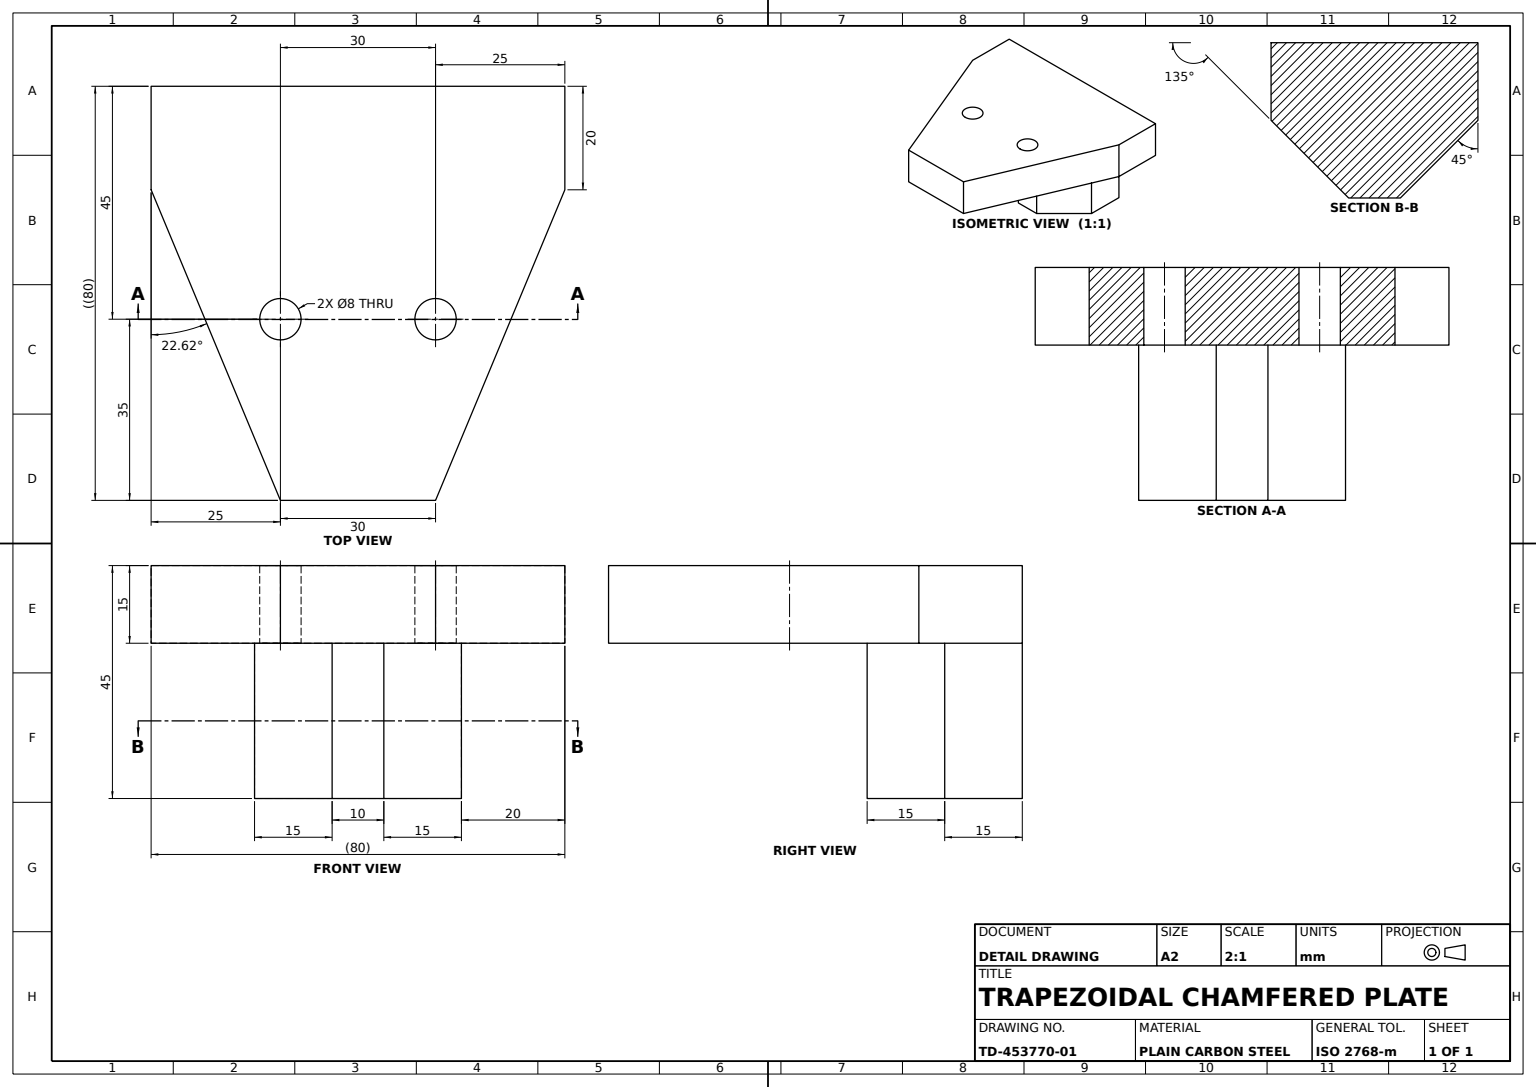
from build123d import *

# Parameters (mm, degrees)
BASE_PLATE_SKETCH_W      = 80
BASE_PLATE_SKETCH_H      = 10
BASE_PLATE_DEPTH         = 20
PENTAGONAL_BOSS_DEPTH    = 15
FOUR_SIDED_BOSS_SKETCH_W = 80
FOUR_SIDED_BOSS_SKETCH_H = 5
FOUR_SIDED_BOSS_DEPTH    = 20
OCTAGONAL_BOSS_DEPTH     = 30
HOLES_2X_8_SKETCH_R      = 4
HOLES_2X_8_DEPTH         = 15


with BuildPart() as part:
    # Base Plate Sketch → Base Plate (new body)
    with BuildSketch(Plane.XY):
        with Locations((40, 5)):
            Rectangle(BASE_PLATE_SKETCH_W, BASE_PLATE_SKETCH_H)
    extrude(amount=BASE_PLATE_DEPTH)

    # Pentagonal Boss Sketch → Pentagonal Boss (add)
    with BuildSketch(Plane.XZ):
        Polygon((40, 80), (25, 80), (0, 20), (80, 20), (55, 80), align=None)
    extrude(amount=-PENTAGONAL_BOSS_DEPTH)

    # Four-Sided Boss Sketch → Four-Sided Boss (add)
    with BuildSketch(Plane(origin=(0, 0, 0), x_dir=(-1, 0, 0), z_dir=(0, 0, -1))):
        with Locations((-40, 12.5)):
            Rectangle(FOUR_SIDED_BOSS_SKETCH_W, FOUR_SIDED_BOSS_SKETCH_H)
    extrude(amount=-FOUR_SIDED_BOSS_DEPTH)

    # Octagonal Boss Sketch → Octagonal Boss (add)
    with BuildSketch(Plane.XZ):
        Polygon((40, 0), (60, 0), (60, 15), (45, 30), (40, 30), (35, 30), (20, 15), (20, 0), align=None)
    extrude(amount=OCTAGONAL_BOSS_DEPTH)

    # Holes 2xØ8 Sketch → Holes 2xØ8 (cut)
    with BuildSketch(Plane.XZ):
        with Locations(Location((25, 45, 0), (0, 0, 270))):
            Circle(HOLES_2X_8_SKETCH_R)
        with Locations(Location((55, 45, 0), (0, 0, 270))):
            Circle(HOLES_2X_8_SKETCH_R)
    extrude(amount=-HOLES_2X_8_DEPTH, mode=Mode.SUBTRACT)


solid = part.part
